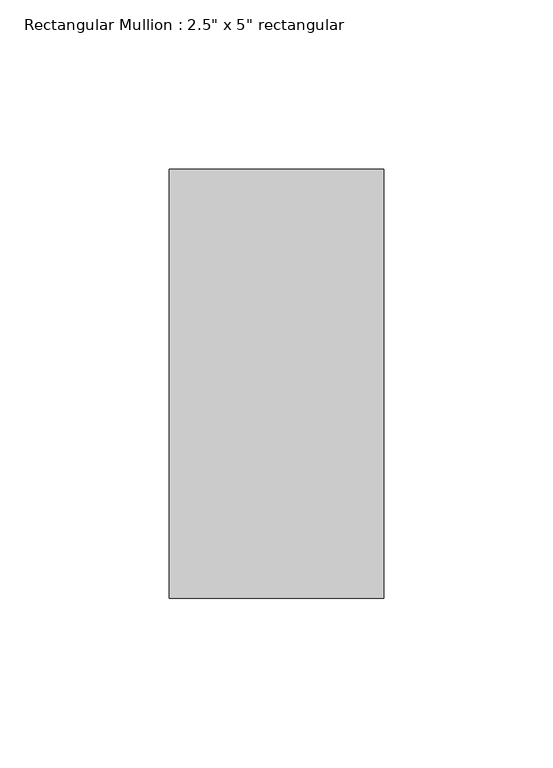
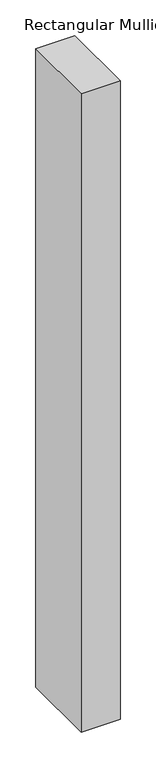
"""IFC4 building model written with IfcOpenShell, lengths in millimetres: member geometry."""

from ifc_helpers import new_model, si_unit, frame, origin, place, context, project, spatial, polyline, outline, extrude, source, transform, mapped, element, save


def member_273a15f2(model_context):
    return source(origin(), model_context, "Body", "SweptSolid", [
        extrude(outline(polyline([(0.0, 63.5), (0.0, -63.5), (-63.5, -63.5), (-63.5, 63.5), (0.0, 63.5)])), frame((0.0, 0.0, -1092.2), z_axis=(0.0, 0.0, 1.0), x_axis=(1.0, 0.0, 0.0)), (0.0, 0.0, 1.0), 1092.2),
    ])


if __name__ == "__main__":
    model = new_model("IFC4")
    model_context = context("Model", 3, world=origin())
    ifc_project = project(units=[si_unit("LENGTHUNIT", "METRE", prefix="MILLI")], contexts=[model_context])
    site = spatial("IfcSite", under=ifc_project)
    building = spatial("IfcBuilding", under=site)
    placement = place(None, origin())
    member_shape = member_273a15f2(model_context)
    element("IfcMember", 1, ObjectType="Rectangular Mullion : 2.5\" x 5\" rectangular", at=placement, inside=building, context=model_context, shape_type="MappedRepresentation", body=[
        mapped(member_shape, transform((0.0, 0.0, 0.0), x_axis=(1.0, 0.0, 0.0), y_axis=(0.0, 1.0, 0.0), z_axis=(0.0, 0.0, 1.0))),
    ])
    save(model, "model.ifc")

# Revit data of these elements
# Type "Rectangular Mullion : 2.5\" x 5\" rectangular"
#   built-in parameter 1007304 = 0.416667 (stored number, unit not read)
#   built-in parameter 1007301 = 0.104167 (stored number, unit not read)
#   built-in parameter 1007300 = 0.104167 (stored number, unit not read)
# Element 1 (IfcMember, "Rectangular Mullion : 2.5\" x 5\" rectangular")
#   Materials on its faces: "Aluminum"
# Materials
#   "Aluminum": class "Metal", colour RGB 247 247 247, transparency 0, Description = "Aluminum 6061", Cost = 0
